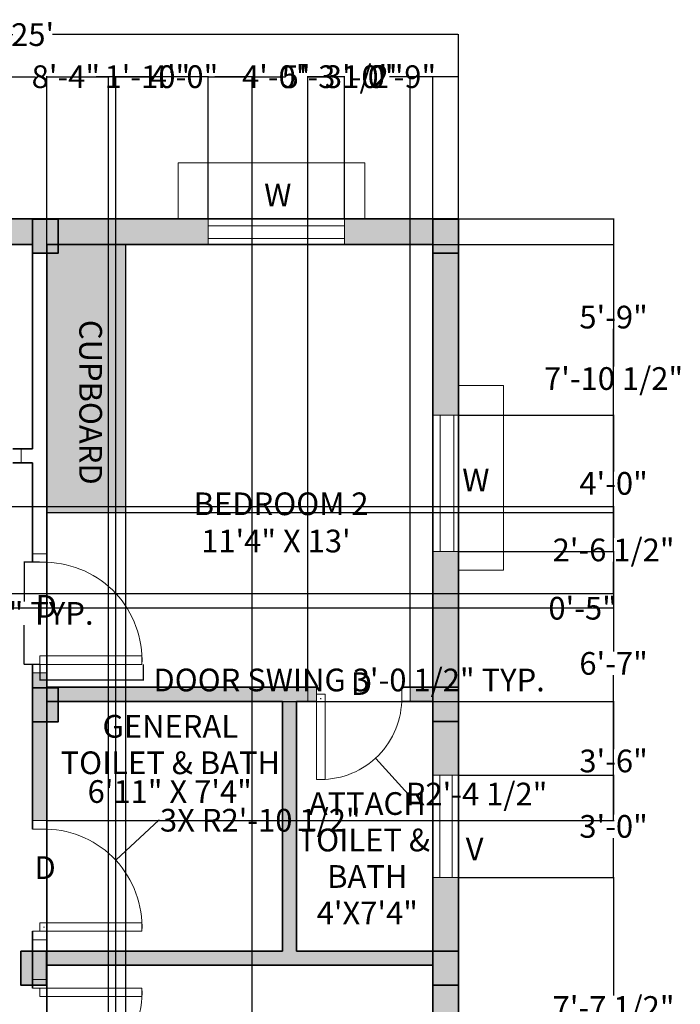
# Model space of a CAD drawing. Units: inches. Extents: x 374 to 1054, y -870 to -188.
# Tile 3 of 3: x 601 to 834, y -535 to -188. Entities that reach past the tile are written whole.
import ezdxf
from ezdxf.enums import TextEntityAlignment as Align

# ---------------------------------------------------------------- set-up
doc = ezdxf.new("R2010")
doc.units = ezdxf.units.IN
doc.header["$MEASUREMENT"] = 0
for name, color, linetype, lineweight, true_color in [('A-ANNO-DIMS', 244, 'Continuous', 18, 0x991b1e), ('A-AREA-IDEN', 116, 'Continuous', 18, 0x136734), ('A-WALL-PATT', 116, 'Continuous', 13, 0x136734)]:
    doc.layers.add(name, color=color, linetype=linetype, lineweight=lineweight, true_color=true_color)
for name, color, linetype, lineweight in [('A-ANNO-TEXT', 7, 'Continuous', 18), ('A-COLS', 1, 'Continuous', 35), ('A-DOOR', 4, 'Continuous', 18), ('A-FLOR-CASE', 8, 'Continuous', 25), ('A-FLOR-CASE-PATT', 8, 'Continuous', 13), ('A-GLAZ', 4, 'Continuous', 18), ('A-GLAZ-PROJ', 4, 'Continuous', 13), ('A-WALL', 7, 'Continuous', 35)]:
    doc.layers.add(name, color=color, linetype=linetype, lineweight=lineweight)
doc.styles.get("Standard").update_dxf_attribs({"font": 'arial.ttf'})
doc.dimstyles.get("Standard").update_dxf_attribs({"dimtxt": 8, "dimasz": 0.18, "dimexe": 0.18, "dimexo": 0.0625, "dimgap": 0.09, "dimtad": 0, "dimtih": 1, "dimtoh": 1, "dimzin": 0, "dimdsep": 46, "dimlunit": 3, "dimtxsty": 'Standard', "dimcen": 0.09, "dimadec": 0, "dimazin": 0, "dimtfac": 1, "dimtofl": 0, "dimtmove": 0, "dimatfit": 3, "dimfxl": 1, "dimtolj": 1, "dimtzin": 0, "dimarcsym": 0})

# ---------------------------------------------------------------- blocks, each defined once
blk = doc.blocks.new('*D1')
at = {"layer": 'A-ANNO-DIMS', "color": 0, "lineweight": -2, "transparency": 16777216}
for p, q in [((455.9, -257.88), (455.9, -192.83)), ((456.08, -193.01), (598.96, -193.01)), ((755.72, -193.01), (612.85, -193.01)), ((755.9, -257.88), (755.9, -192.83))]:
    blk.add_line(p, q, dxfattribs=at)
at = {"layer": 'A-ANNO-DIMS', "color": 0, "transparency": 16777216}
for points in [[(456.08, -192.98), (456.08, -193.04), (455.9, -193.01)], [(755.72, -192.98), (755.72, -193.04), (755.9, -193.01)]]:
    blk.add_solid(points, dxfattribs=at)
at = {"layer": 'Defpoints', "color": 0, "transparency": 16777216}
for p in [(755.9, -193.01), (455.9, -257.94), (755.9, -257.94)]:
    blk.add_point(p, dxfattribs=at)
at = {"layer": 'A-ANNO-DIMS', "color": 0, "transparency": 16777216, "insert": (605.9, -193.01), "char_height": 8, "attachment_point": 5}
blk.add_mtext("\\A1;25'", dxfattribs=at)
blk = doc.blocks.new('COL-12X9')
h = blk.add_hatch(color=256)
h.dxf.hatch_style = 1
h.paths.add_polyline_path([(6, 4.5), (-6, 4.5), (-6, -4.5), (6, -4.5)])
blk.add_lwpolyline([(-6, 4.5), (6, 4.5), (6, -4.5), (-6, -4.5)], close=True)
blk = doc.blocks.new('DOOR-SWING-36')
blk.add_lwpolyline([(0, 0), (-3, 0), (-3, 36), (0, 36)], close=True)
blk.add_arc((-1.5, 1.52), 34.51, 87.5091, 178.3707)
blk = doc.blocks.new('*D8')
at = {"layer": 'A-ANNO-DIMS', "color": 0, "lineweight": -2, "transparency": 16777216}
for p, q in [((608.4, -415), (608.4, -420.58)), ((644.81, -415), (644.81, -420.58)), ((608.58, -420.4), (644.63, -420.4)), ((644.81, -420.4), (644.99, -420.4))]:
    blk.add_line(p, q, dxfattribs=at)
at = {"layer": 'A-ANNO-DIMS', "color": 0, "transparency": 16777216}
for points in [[(608.58, -420.37), (608.58, -420.43), (608.4, -420.4)], [(644.63, -420.37), (644.63, -420.43), (644.81, -420.4)]]:
    blk.add_solid(points, dxfattribs=at)
at = {"layer": 'Defpoints', "color": 0, "transparency": 16777216}
for p in [(608.4, -414.94), (644.81, -414.94), (644.81, -420.4)]:
    blk.add_point(p, dxfattribs=at)
at = {"layer": 'A-ANNO-DIMS', "color": 0, "transparency": 16777216, "insert": (717.38, -420.4), "char_height": 8, "attachment_point": 5}
blk.add_mtext('\\A1;DOOR SWING 3\'-0 1/2" TYP.', dxfattribs=at)
blk = doc.blocks.new('*D9')
at = {"layer": 'A-ANNO-DIMS', "color": 0, "lineweight": -2, "transparency": 16777216}
for p, q in [((608.34, -378.94), (602.76, -378.94)), ((602.94, -379.12), (602.94, -392.76)), ((602.94, -414.76), (602.94, -401.12)), ((608.34, -414.94), (602.76, -414.94))]:
    blk.add_line(p, q, dxfattribs=at)
at = {"layer": 'A-ANNO-DIMS', "color": 0, "transparency": 16777216}
for points in [[(602.91, -379.12), (602.97, -379.12), (602.94, -378.94)], [(602.91, -414.76), (602.97, -414.76), (602.94, -414.94)]]:
    blk.add_solid(points, dxfattribs=at)
at = {"layer": 'Defpoints', "color": 0, "transparency": 16777216}
for p in [(608.4, -378.94), (602.94, -414.94), (608.4, -414.94)]:
    blk.add_point(p, dxfattribs=at)
at = {"layer": 'A-ANNO-DIMS', "color": 0, "transparency": 16777216, "insert": (602.94, -396.94), "char_height": 8, "attachment_point": 5}
blk.add_mtext('\\A1;3\'-0" TYP.', dxfattribs=at)
blk = doc.blocks.new('*D14')
at = {"layer": 'A-ANNO-DIMS', "color": 0, "lineweight": -2, "transparency": 16777216}
for p, q in [((567.48, -257.88), (567.48, -207.66)), ((567.66, -207.84), (606.87, -207.84)), ((667.53, -207.84), (628.32, -207.84)), ((667.71, -257.88), (667.71, -207.66))]:
    blk.add_line(p, q, dxfattribs=at)
at = {"layer": 'A-ANNO-DIMS', "color": 0, "transparency": 16777216}
for points in [[(567.66, -207.81), (567.66, -207.87), (567.48, -207.84)], [(667.53, -207.81), (667.53, -207.87), (667.71, -207.84)]]:
    blk.add_solid(points, dxfattribs=at)
at = {"layer": 'Defpoints', "color": 0, "transparency": 16777216}
for p in [(667.71, -207.84), (567.48, -257.94), (667.71, -257.94)]:
    blk.add_point(p, dxfattribs=at)
at = {"layer": 'A-ANNO-DIMS', "color": 0, "transparency": 16777216, "insert": (617.6, -207.84), "char_height": 8, "attachment_point": 5}
blk.add_mtext('\\A1;8\'-4"', dxfattribs=at)
blk = doc.blocks.new('*D15')
at = {"layer": 'A-ANNO-DIMS', "color": 0, "lineweight": -2, "transparency": 16777216}
for p, q in [((667.71, -257.88), (667.71, -207.66)), ((667.89, -207.84), (680.83, -207.84)), ((715.53, -207.84), (702.59, -207.84)), ((715.71, -257.88), (715.71, -207.66))]:
    blk.add_line(p, q, dxfattribs=at)
at = {"layer": 'A-ANNO-DIMS', "color": 0, "transparency": 16777216}
for points in [[(667.89, -207.81), (667.89, -207.87), (667.71, -207.84)], [(715.53, -207.81), (715.53, -207.87), (715.71, -207.84)]]:
    blk.add_solid(points, dxfattribs=at)
at = {"layer": 'Defpoints', "color": 0, "transparency": 16777216}
for p in [(715.71, -207.84), (667.71, -257.94), (715.71, -257.94)]:
    blk.add_point(p, dxfattribs=at)
at = {"layer": 'A-ANNO-DIMS', "color": 0, "transparency": 16777216, "insert": (691.71, -207.84), "char_height": 8, "attachment_point": 5}
blk.add_mtext('\\A1;4\'-0"', dxfattribs=at)
blk = doc.blocks.new('*D24')
at = {"layer": 'A-ANNO-DIMS', "color": 0, "lineweight": -2, "transparency": 16777216}
for p, q in [((746.9, -207.84), (746.72, -207.84)), ((746.9, -266.88), (746.9, -207.66)), ((755.72, -207.84), (747.08, -207.84)), ((755.9, -257.88), (755.9, -207.66))]:
    blk.add_line(p, q, dxfattribs=at)
at = {"layer": 'A-ANNO-DIMS', "color": 0, "transparency": 16777216}
for points in [[(747.08, -207.81), (747.08, -207.87), (746.9, -207.84)], [(755.72, -207.81), (755.72, -207.87), (755.9, -207.84)]]:
    blk.add_solid(points, dxfattribs=at)
at = {"layer": 'Defpoints', "color": 0, "transparency": 16777216}
for p in [(746.9, -207.84), (755.9, -257.94), (746.9, -266.94)]:
    blk.add_point(p, dxfattribs=at)
at = {"layer": 'A-ANNO-DIMS', "color": 0, "transparency": 16777216, "insert": (736, -207.84), "char_height": 8, "attachment_point": 5}
blk.add_mtext('\\A1;0\'-9"', dxfattribs=at)
blk = doc.blocks.new('*D25')
at = {"layer": 'A-ANNO-DIMS', "color": 0, "lineweight": -2, "transparency": 16777216}
for p, q in [((541.93, -389.94), (810.73, -389.94)), ((810.55, -390.12), (810.55, -394.76)), ((541.92, -394.94), (810.73, -394.94)), ((810.55, -395.12), (810.37, -395.12)), ((810.55, -394.94), (810.55, -395.12))]:
    blk.add_line(p, q, dxfattribs=at)
at = {"layer": 'A-ANNO-DIMS', "color": 0, "transparency": 16777216}
for points in [[(810.52, -390.12), (810.58, -390.12), (810.55, -389.94)], [(810.52, -394.76), (810.58, -394.76), (810.55, -394.94)]]:
    blk.add_solid(points, dxfattribs=at)
at = {"layer": 'Defpoints', "color": 0, "transparency": 16777216}
for p in [(541.86, -389.94), (541.86, -394.94), (810.55, -394.94)]:
    blk.add_point(p, dxfattribs=at)
at = {"layer": 'A-ANNO-DIMS', "color": 0, "transparency": 16777216, "insert": (799.65, -395.12), "char_height": 8, "attachment_point": 5}
blk.add_mtext('\\A1;0\'-5"', dxfattribs=at)
blk = doc.blocks.new('*D26')
at = {"layer": 'A-ANNO-DIMS', "color": 0, "lineweight": -2, "transparency": 16777216}
for p, q in [((755.97, -257.94), (810.73, -257.94)), ((810.55, -258.12), (810.55, -288.36)), ((810.55, -326.96), (810.55, -296.71)), ((755.97, -327.14), (810.73, -327.14))]:
    blk.add_line(p, q, dxfattribs=at)
at = {"layer": 'A-ANNO-DIMS', "color": 0, "transparency": 16777216}
for points in [[(810.52, -258.12), (810.58, -258.12), (810.55, -257.94)], [(810.52, -326.96), (810.58, -326.96), (810.55, -327.14)]]:
    blk.add_solid(points, dxfattribs=at)
at = {"layer": 'Defpoints', "color": 0, "transparency": 16777216}
for p in [(755.9, -257.94), (755.9, -327.14), (810.55, -327.14)]:
    blk.add_point(p, dxfattribs=at)
at = {"layer": 'A-ANNO-DIMS', "color": 0, "transparency": 16777216, "insert": (810.55, -292.54), "char_height": 8, "attachment_point": 5}
blk.add_mtext('\\A1;5\'-9"', dxfattribs=at)
blk = doc.blocks.new('*D27')
at = {"layer": 'A-ANNO-DIMS', "color": 0, "lineweight": -2, "transparency": 16777216}
for p, q in [((755.97, -327.14), (810.73, -327.14)), ((810.55, -327.32), (810.55, -346.96)), ((810.55, -374.96), (810.55, -355.31)), ((755.97, -375.14), (810.73, -375.14))]:
    blk.add_line(p, q, dxfattribs=at)
at = {"layer": 'A-ANNO-DIMS', "color": 0, "transparency": 16777216}
for points in [[(810.52, -327.32), (810.58, -327.32), (810.55, -327.14)], [(810.52, -374.96), (810.58, -374.96), (810.55, -375.14)]]:
    blk.add_solid(points, dxfattribs=at)
at = {"layer": 'Defpoints', "color": 0, "transparency": 16777216}
for p in [(755.9, -327.14), (755.9, -375.14), (810.55, -375.14)]:
    blk.add_point(p, dxfattribs=at)
at = {"layer": 'A-ANNO-DIMS', "color": 0, "transparency": 16777216, "insert": (810.55, -351.14), "char_height": 8, "attachment_point": 5}
blk.add_mtext('\\A1;4\'-0"', dxfattribs=at)
blk = doc.blocks.new('*D28')
at = {"layer": 'A-ANNO-DIMS', "color": 0, "lineweight": -2, "transparency": 16777216}
for p, q in [((755.97, -375.14), (810.73, -375.14)), ((810.55, -375.32), (810.55, -410.39)), ((810.55, -453.81), (810.55, -418.74)), ((755.97, -453.99), (810.73, -453.99))]:
    blk.add_line(p, q, dxfattribs=at)
at = {"layer": 'A-ANNO-DIMS', "color": 0, "transparency": 16777216}
for points in [[(810.52, -375.32), (810.58, -375.32), (810.55, -375.14)], [(810.52, -453.81), (810.58, -453.81), (810.55, -453.99)]]:
    blk.add_solid(points, dxfattribs=at)
at = {"layer": 'Defpoints', "color": 0, "transparency": 16777216}
for p in [(755.9, -375.14), (755.9, -453.99), (810.55, -453.99)]:
    blk.add_point(p, dxfattribs=at)
at = {"layer": 'A-ANNO-DIMS', "color": 0, "transparency": 16777216, "insert": (810.55, -414.57), "char_height": 8, "attachment_point": 5}
blk.add_mtext('\\A1;6\'-7"', dxfattribs=at)
blk = doc.blocks.new('*D29')
at = {"layer": 'A-ANNO-DIMS', "color": 0, "lineweight": -2, "transparency": 16777216}
for p, q in [((755.97, -453.99), (810.73, -453.99)), ((810.55, -454.17), (810.55, -467.82)), ((810.55, -489.81), (810.55, -476.17)), ((755.97, -489.99), (810.73, -489.99))]:
    blk.add_line(p, q, dxfattribs=at)
at = {"layer": 'A-ANNO-DIMS', "color": 0, "transparency": 16777216}
for points in [[(810.52, -454.17), (810.58, -454.17), (810.55, -453.99)], [(810.52, -489.81), (810.58, -489.81), (810.55, -489.99)]]:
    blk.add_solid(points, dxfattribs=at)
at = {"layer": 'Defpoints', "color": 0, "transparency": 16777216}
for p in [(755.9, -453.99), (755.9, -489.99), (810.55, -489.99)]:
    blk.add_point(p, dxfattribs=at)
at = {"layer": 'A-ANNO-DIMS', "color": 0, "transparency": 16777216, "insert": (810.55, -471.99), "char_height": 8, "attachment_point": 5}
blk.add_mtext('\\A1;3\'-0"', dxfattribs=at)
blk = doc.blocks.new('*D30')
at = {"layer": 'A-ANNO-DIMS', "color": 0, "lineweight": -2, "transparency": 16777216}
for p, q in [((755.97, -489.99), (810.73, -489.99)), ((810.55, -490.17), (810.55, -531.58)), ((810.55, -581.43), (810.55, -540.03)), ((755.97, -581.61), (810.73, -581.61))]:
    blk.add_line(p, q, dxfattribs=at)
at = {"layer": 'A-ANNO-DIMS', "color": 0, "transparency": 16777216}
for points in [[(810.52, -490.17), (810.58, -490.17), (810.55, -489.99)], [(810.52, -581.43), (810.58, -581.43), (810.55, -581.61)]]:
    blk.add_solid(points, dxfattribs=at)
at = {"layer": 'Defpoints', "color": 0, "transparency": 16777216}
for p in [(755.9, -489.99), (755.9, -581.61), (810.55, -581.61)]:
    blk.add_point(p, dxfattribs=at)
at = {"layer": 'A-ANNO-DIMS', "color": 0, "transparency": 16777216, "insert": (810.55, -535.8), "char_height": 8, "attachment_point": 5}
blk.add_mtext('\\A1;7\'-7 1/2"', dxfattribs=at)
blk = doc.blocks.new('*D35')
at = {"layer": 'A-ANNO-DIMS', "color": 0, "lineweight": -2, "transparency": 16777216}
for p, q in [((610.9, -361.5), (610.9, -822.55)), ((638.56, -361.5), (638.56, -822.55)), ((611.08, -822.37), (638.38, -822.37)), ((638.56, -822.37), (638.74, -822.37))]:
    blk.add_line(p, q, dxfattribs=at)
at = {"layer": 'A-ANNO-DIMS', "color": 0, "transparency": 16777216}
for points in [[(611.08, -822.34), (611.08, -822.4), (610.9, -822.37)], [(638.38, -822.34), (638.38, -822.4), (638.56, -822.37)]]:
    blk.add_solid(points, dxfattribs=at)
at = {"layer": 'Defpoints', "color": 0, "transparency": 16777216}
for p in [(610.9, -361.44), (638.56, -361.44), (638.56, -822.37)]:
    blk.add_point(p, dxfattribs=at)
at = {"layer": 'A-ANNO-DIMS', "color": 0, "transparency": 16777216, "insert": (658.85, -822.37), "char_height": 8, "attachment_point": 5}
blk.add_mtext('\\A1;2\'-3 1/2"', dxfattribs=at)
blk = doc.blocks.new('*D36')
at = {"layer": 'A-ANNO-DIMS', "color": 0, "lineweight": -2, "transparency": 16777216}
for p, q in [((638.63, -266.94), (810.73, -266.94)), ((810.55, -267.12), (810.55, -309.96)), ((810.55, -361.26), (810.55, -318.41)), ((638.63, -361.44), (810.73, -361.44))]:
    blk.add_line(p, q, dxfattribs=at)
at = {"layer": 'A-ANNO-DIMS', "color": 0, "transparency": 16777216}
for points in [[(810.52, -267.12), (810.58, -267.12), (810.55, -266.94)], [(810.52, -361.26), (810.58, -361.26), (810.55, -361.44)]]:
    blk.add_solid(points, dxfattribs=at)
at = {"layer": 'Defpoints', "color": 0, "transparency": 16777216}
for p in [(638.56, -266.94), (810.55, -266.94), (638.56, -361.44)]:
    blk.add_point(p, dxfattribs=at)
at = {"layer": 'A-ANNO-DIMS', "color": 0, "transparency": 16777216, "insert": (810.55, -314.19), "char_height": 8, "attachment_point": 5}
blk.add_mtext('\\A1;7\'-10 1/2"', dxfattribs=at)
blk = doc.blocks.new('*D37')
at = {"layer": 'A-ANNO-DIMS', "color": 0, "lineweight": -2, "transparency": 16777216}
for p, q in [((610.9, -588.25), (610.9, -207.66)), ((611.08, -207.84), (632.5, -207.84)), ((632.68, -588.25), (632.68, -207.66)), ((632.68, -207.84), (632.86, -207.84))]:
    blk.add_line(p, q, dxfattribs=at)
at = {"layer": 'A-ANNO-DIMS', "color": 0, "transparency": 16777216}
for points in [[(611.08, -207.81), (611.08, -207.87), (610.9, -207.84)], [(632.5, -207.81), (632.5, -207.87), (632.68, -207.84)]]:
    blk.add_solid(points, dxfattribs=at)
at = {"layer": 'Defpoints', "color": 0, "transparency": 16777216}
for p in [(632.68, -207.84), (610.9, -588.31), (632.68, -588.31)]:
    blk.add_point(p, dxfattribs=at)
at = {"layer": 'A-ANNO-DIMS', "color": 0, "transparency": 16777216, "insert": (646.31, -207.84), "char_height": 8, "attachment_point": 5}
blk.add_mtext('\\A1;1\'-10"', dxfattribs=at)
blk = doc.blocks.new('*D43')
at = {"layer": 'A-ANNO-DIMS', "color": 0, "lineweight": -2, "transparency": 16777216}
for p, q in [((635.25, -680.88), (635.25, -207.66)), ((635.43, -207.84), (648.36, -207.84)), ((683.07, -207.84), (670.13, -207.84)), ((683.25, -680.88), (683.25, -207.66))]:
    blk.add_line(p, q, dxfattribs=at)
at = {"layer": 'A-ANNO-DIMS', "color": 0, "transparency": 16777216}
for points in [[(635.43, -207.81), (635.43, -207.87), (635.25, -207.84)], [(683.07, -207.81), (683.07, -207.87), (683.25, -207.84)]]:
    blk.add_solid(points, dxfattribs=at)
at = {"layer": 'Defpoints', "color": 0, "transparency": 16777216}
for p in [(683.25, -207.84), (635.25, -680.94), (683.25, -680.94)]:
    blk.add_point(p, dxfattribs=at)
at = {"layer": 'A-ANNO-DIMS', "color": 0, "transparency": 16777216, "insert": (659.25, -207.84), "char_height": 8, "attachment_point": 5}
blk.add_mtext('\\A1;4\'-0"', dxfattribs=at)
blk = doc.blocks.new('*D44')
at = {"layer": 'A-ANNO-DIMS', "color": 0, "lineweight": -2, "transparency": 16777216}
for p, q in [((683.25, -680.88), (683.25, -207.66)), ((683.43, -207.84), (695.03, -207.84)), ((746.72, -207.84), (735.12, -207.84)), ((746.9, -680.88), (746.9, -207.66))]:
    blk.add_line(p, q, dxfattribs=at)
at = {"layer": 'A-ANNO-DIMS', "color": 0, "transparency": 16777216}
for points in [[(683.43, -207.81), (683.43, -207.87), (683.25, -207.84)], [(746.72, -207.81), (746.72, -207.87), (746.9, -207.84)]]:
    blk.add_solid(points, dxfattribs=at)
at = {"layer": 'Defpoints', "color": 0, "transparency": 16777216}
for p in [(746.9, -207.84), (683.25, -680.94), (746.9, -680.94)]:
    blk.add_point(p, dxfattribs=at)
at = {"layer": 'A-ANNO-DIMS', "color": 0, "transparency": 16777216, "insert": (715.08, -207.84), "char_height": 8, "attachment_point": 5}
blk.add_mtext('\\A1;5\'-3 1/2"', dxfattribs=at)
blk = doc.blocks.new('*D46')
at = {"layer": 'A-ANNO-DIMS', "color": 0, "lineweight": -2, "transparency": 16777216}
for p, q in [((541.95, -359.22), (810.73, -359.22)), ((810.55, -359.4), (810.55, -370.35)), ((810.55, -389.76), (810.55, -378.81)), ((541.93, -389.94), (810.73, -389.94))]:
    blk.add_line(p, q, dxfattribs=at)
at = {"layer": 'A-ANNO-DIMS', "color": 0, "transparency": 16777216}
for points in [[(810.52, -359.4), (810.58, -359.4), (810.55, -359.22)], [(810.52, -389.76), (810.58, -389.76), (810.55, -389.94)]]:
    blk.add_solid(points, dxfattribs=at)
at = {"layer": 'Defpoints', "color": 0, "transparency": 16777216}
for p in [(541.89, -359.22), (541.86, -389.94), (810.55, -389.94)]:
    blk.add_point(p, dxfattribs=at)
at = {"layer": 'A-ANNO-DIMS', "color": 0, "transparency": 16777216, "insert": (810.55, -374.58), "char_height": 8, "attachment_point": 5}
blk.add_mtext('\\A1;2\'-6 1/2"', dxfattribs=at)
blk = doc.blocks.new('*D47')
at = {"layer": 'A-ANNO-DIMS', "color": 0, "lineweight": -2, "transparency": 16777216}
for p, q in [((702.9, -422.88), (702.9, -207.66)), ((703.08, -207.84), (710.18, -207.84)), ((738.72, -207.84), (731.63, -207.84)), ((738.9, -422.88), (738.9, -207.66))]:
    blk.add_line(p, q, dxfattribs=at)
at = {"layer": 'A-ANNO-DIMS', "color": 0, "transparency": 16777216}
for points in [[(703.08, -207.81), (703.08, -207.87), (702.9, -207.84)], [(738.72, -207.81), (738.72, -207.87), (738.9, -207.84)]]:
    blk.add_solid(points, dxfattribs=at)
at = {"layer": 'Defpoints', "color": 0, "transparency": 16777216}
for p in [(738.9, -207.84), (702.9, -422.94), (738.9, -422.94)]:
    blk.add_point(p, dxfattribs=at)
at = {"layer": 'A-ANNO-DIMS', "color": 0, "transparency": 16777216, "insert": (720.9, -207.84), "char_height": 8, "attachment_point": 5}
blk.add_mtext('\\A1;3\'-0"', dxfattribs=at)
blk = doc.blocks.new('*D48')
at = {"layer": 'A-ANNO-DIMS', "color": 0, "lineweight": -2, "transparency": 16777216}
for p, q in [((610.97, -427.94), (810.73, -427.94)), ((810.55, -428.12), (810.55, -444.76)), ((810.55, -469.76), (810.55, -453.12)), ((610.97, -469.94), (810.73, -469.94))]:
    blk.add_line(p, q, dxfattribs=at)
at = {"layer": 'A-ANNO-DIMS', "color": 0, "transparency": 16777216}
for points in [[(810.52, -428.12), (810.58, -428.12), (810.55, -427.94)], [(810.52, -469.76), (810.58, -469.76), (810.55, -469.94)]]:
    blk.add_solid(points, dxfattribs=at)
at = {"layer": 'Defpoints', "color": 0, "transparency": 16777216}
for p in [(610.9, -427.94), (610.9, -469.94), (810.55, -469.94)]:
    blk.add_point(p, dxfattribs=at)
at = {"layer": 'A-ANNO-DIMS', "color": 0, "transparency": 16777216, "insert": (810.55, -448.94), "char_height": 8, "attachment_point": 5}
blk.add_mtext('\\A1;3\'-6"', dxfattribs=at)
blk = doc.blocks.new('*D51')
at = {"layer": 'A-ANNO-DIMS', "color": 0, "lineweight": -2, "transparency": 16777216}
for p, q in [((650.35, -469.82), (635.32, -483.8)), ((650.53, -469.82), (650.35, -469.82)), ((609.83, -507.44), (610.01, -507.44)), ((609.92, -507.53), (609.92, -507.35))]:
    blk.add_line(p, q, dxfattribs=at)
at = {"layer": 'A-ANNO-DIMS', "color": 0, "transparency": 16777216}
blk.add_solid([(635.3, -483.78), (635.34, -483.83), (635.19, -483.93)], dxfattribs=at)
at = {"layer": 'Defpoints', "color": 0, "transparency": 16777216}
for p in [(635.19, -483.93), (609.92, -507.44)]:
    blk.add_point(p, dxfattribs=at)
at = {"layer": 'A-ANNO-DIMS', "color": 0, "transparency": 16777216, "insert": (686.1, -469.82), "char_height": 8, "attachment_point": 5}
blk.add_mtext('\\A1;3X R2\'-10 1/2"', dxfattribs=at)
blk = doc.blocks.new('*D52')
at = {"layer": 'A-ANNO-DIMS', "color": 0, "lineweight": -2, "transparency": 16777216}
for p, q in [((707.31, -426.96), (707.49, -426.96)), ((707.4, -427.05), (707.4, -426.87)), ((738.24, -460.59), (726.8, -448.11)), ((738.42, -460.59), (738.24, -460.59))]:
    blk.add_line(p, q, dxfattribs=at)
at = {"layer": 'A-ANNO-DIMS', "color": 0, "transparency": 16777216}
blk.add_solid([(726.82, -448.09), (726.77, -448.14), (726.67, -447.98)], dxfattribs=at)
at = {"layer": 'Defpoints', "color": 0, "transparency": 16777216}
for p in [(707.4, -426.96), (726.67, -447.98)]:
    blk.add_point(p, dxfattribs=at)
at = {"layer": 'A-ANNO-DIMS', "color": 0, "transparency": 16777216, "insert": (762.29, -460.59), "char_height": 8, "attachment_point": 5}
blk.add_mtext('\\A1;R2\'-4 1/2"', dxfattribs=at)

msp = doc.modelspace()

# ---------------------------------------------------------------- hatches: boundary and pattern name
at = {"layer": 'A-FLOR-CASE-PATT'}
h = msp.add_hatch(dxfattribs=at)
h.set_pattern_fill('AR-HBONE', color=256)
h.paths.add_polyline_path([(638.563, -266.938), (610.905, -266.938), (610.905, -343.938), (610.905, -361.438), (638.563, -361.438)])
h.paths.add_polyline_path([(620.136, -288.822), (620.136, -356.301), (632.553, -356.301), (632.553, -288.822)], flags=24)
h.paths.add_polyline_path([(727.152, -700.465), (727.152, -761.497), (739.414, -761.497), (739.414, -700.465)], flags=9)
h.paths.add_polyline_path([(497.837, -702.053), (512.386, -702.053), (512.386, -690.053), (497.837, -690.053)], flags=9)
h.paths.add_polyline_path([(494.709, -751.886), (551.702, -751.886), (551.702, -739.837), (494.709, -739.837)], flags=9)
h.paths.add_polyline_path([(490.155, -739.027), (556.256, -739.027), (556.256, -727.027), (490.155, -727.027)], flags=9)
h.paths.add_polyline_path([(488.741, -637.8), (555.988, -637.8), (555.988, -625.538), (488.741, -625.538)], flags=9)
h.paths.add_polyline_path([(501.975, -624.968), (542.755, -624.968), (542.755, -612.559), (501.975, -612.559)], flags=9)
h.paths.add_polyline_path([(498.568, -470.79), (565.812, -470.79), (565.812, -458.536), (498.568, -458.536)], flags=9)
h.paths.add_polyline_path([(510.563, -457.965), (553.816, -457.965), (553.816, -445.555), (510.563, -445.555)], flags=9)
h.paths.add_polyline_path([(474.841, -376.354), (525.689, -376.354), (525.689, -364.092), (474.841, -364.092)], flags=9)
h.paths.add_polyline_path([(483.939, -363.488), (516.591, -363.488), (516.591, -351.283), (483.939, -351.283)], flags=9)
h.paths.add_polyline_path([(652.121, -604.662), (719.368, -604.662), (719.368, -592.4), (652.121, -592.4)], flags=9)
h.paths.add_polyline_path([(650.141, -591.831), (721.347, -591.831), (721.347, -579.414), (650.141, -579.414)], flags=9)
h.paths.add_polyline_path([(613.577, -603.955), (613.577, -672.673), (625.995, -672.673), (625.995, -603.955)], flags=9)
h.paths.add_polyline_path([(704.619, -508.492), (742.954, -508.492), (742.954, -496.492), (704.619, -496.492)], flags=9)
h.paths.add_polyline_path([(706.883, -495.641), (740.69, -495.641), (740.69, -483.641), (706.883, -483.641)], flags=9)
h.paths.add_polyline_path([(695.312, -483.057), (752.261, -483.057), (752.261, -470.566), (695.312, -470.566)], flags=9)
h.paths.add_polyline_path([(699.358, -470.143), (748.215, -470.143), (748.215, -457.734), (699.358, -457.734)], flags=9)
h.paths.add_polyline_path([(623.681, -465.885), (684.71, -465.885), (684.71, -453.631), (623.681, -453.631)], flags=9)
h.paths.add_polyline_path([(611.019, -455.848), (697.775, -455.848), (697.775, -443.357), (611.019, -443.357)], flags=9)
h.paths.add_polyline_path([(625.622, -442.934), (683.172, -442.934), (683.172, -430.525), (625.622, -430.525)], flags=9)
at = {"layer": 'A-WALL-PATT'}
h = msp.add_hatch(color=256, dxfattribs=at)
h.dxf.hatch_style = 1
h.paths.add_polyline_path([(667.71, -257.938), (614.905, -257.938), (614.905, -266.938), (667.71, -266.938)])
h.paths.add_polyline_path([(746.905, -257.938), (715.71, -257.938), (715.71, -266.938), (746.905, -266.938)])
h.paths.add_polyline_path([(755.905, -270.034), (746.905, -270.034), (746.905, -327.137), (755.905, -327.137)])
h.paths.add_polyline_path([(755.905, -375.137), (746.905, -375.137), (746.905, -422.975), (755.905, -422.975)])
h.paths.add_polyline_path([(605.905, -257.938), (567.481, -257.938), (567.481, -266.938), (605.905, -266.938)])
h.paths.add_polyline_path([(519.481, -257.938), (464.905, -257.938), (464.905, -266.938), (519.481, -266.938)])
h.paths.add_polyline_path([(464.905, -270.108), (455.905, -270.108), (455.905, -285.73), (464.905, -285.73)])
h.paths.add_polyline_path([(464.905, -343.938), (559.905, -343.938), (559.905, -338.938), (464.905, -338.938), (464.905, -333.73), (455.905, -333.73), (455.905, -353.908), (464.905, -353.908)])
h.paths.add_polyline_path([(464.905, -394.938), (541.859, -394.938), (541.863, -389.942), (536.905, -389.938), (464.905, -389.938), (455.905, -389.908), (455.905, -423.118), (464.905, -423.118)])
h.paths.add_polyline_path([(464.905, -435.118), (455.905, -435.118), (455.905, -449.434), (464.905, -449.434)])
h.paths.add_polyline_path([(464.905, -497.434), (455.905, -497.434), (455.905, -515.926), (464.905, -515.926)])
h.paths.add_polyline_path([(464.905, -527.926), (455.905, -527.926), (455.905, -558.14), (464.905, -558.14)])
h.paths.add_polyline_path([(755.905, -489.995), (746.905, -489.995), (746.905, -515.947), (755.905, -515.947)])
h.paths.add_polyline_path([(755.905, -434.975), (746.905, -434.975), (746.905, -453.995), (755.905, -453.995)])
h.paths.add_polyline_path([(746.905, -422.938), (738.905, -422.938), (738.905, -427.938), (746.905, -427.938)])
h.paths.add_polyline_path([(614.905, -423.118), (614.905, -435.118), (605.905, -435.118), (605.905, -423.118), (605.905, -417.938), (610.905, -417.938), (610.905, -423.118)])
h.paths.add_polyline_path([(610.905, -435.118), (605.905, -435.118), (605.905, -469.938), (610.905, -469.938)])
h.paths.add_polyline_path([(541.859, -515.938), (464.905, -515.938), (464.905, -520.938), (541.859, -520.938)])
h.paths.add_polyline_path([(755.905, -527.947), (746.905, -527.947), (746.905, -581.613), (755.905, -581.613)])
h.paths.add_polyline_path([(755.905, -629.613), (746.905, -629.613), (746.905, -677.938), (755.905, -677.938)])
h.paths.add_polyline_path([(755.905, -689.938), (746.905, -689.938), (746.905, -764.938), (755.905, -764.938)])
h.paths.add_polyline_path([(746.905, -680.938), (683.247, -680.938), (683.247, -689.938), (746.905, -689.938)])
h.paths.add_polyline_path([(743.737, -764.938), (701.105, -764.938), (701.105, -773.938), (743.737, -773.938)])
h.paths.add_polyline_path([(653.105, -764.938), (617.905, -764.938), (617.905, -773.938), (653.105, -773.938)])
h.paths.add_polyline_path([(635.247, -680.938), (614.944, -680.938), (614.944, -689.938), (635.247, -689.938)])
h.paths.add_polyline_path([(610.905, -567.938), (605.905, -567.938), (605.905, -677.938), (610.905, -677.938)])
h.paths.add_polyline_path([(558.905, -680.938), (529.314, -680.938), (529.314, -687.485), (529.314, -689.938), (558.905, -689.938)])
h.paths.add_polyline_path([(481.314, -680.938), (464.905, -680.938), (464.905, -689.938), (481.314, -689.938)])
h.paths.add_polyline_path([(464.905, -606.14), (455.905, -606.14), (455.905, -677.938), (464.905, -677.938)])
h.paths.add_polyline_path([(601.753, -550.416), (613.824, -550.416), (613.824, -538.416), (601.753, -538.416)], flags=9)
h.paths.add_polyline_path([(604.254, -492.526), (616.325, -492.526), (616.325, -480.526), (604.254, -480.526)], flags=9)
h.paths.add_polyline_path([(604.661, -400.451), (616.732, -400.451), (616.732, -388.451), (604.661, -388.451)], flags=9)
h.paths.add_polyline_path([(533.025, -378.901), (545.096, -378.901), (545.096, -366.901), (533.025, -366.901)], flags=9)
h.paths.add_polyline_path([(575.128, -346.003), (587.199, -346.003), (587.199, -334.003), (575.128, -334.003)], flags=9)
h.paths.add_polyline_path([(488.741, -637.8), (555.988, -637.8), (555.988, -625.538), (488.741, -625.538)], flags=9)
h.paths.add_polyline_path([(501.975, -624.968), (542.755, -624.968), (542.755, -612.559), (501.975, -612.559)], flags=9)
h.paths.add_polyline_path([(498.568, -470.79), (565.812, -470.79), (565.812, -458.536), (498.568, -458.536)], flags=9)
h.paths.add_polyline_path([(510.563, -457.965), (553.816, -457.965), (553.816, -445.555), (510.563, -445.555)], flags=9)
h.paths.add_polyline_path([(474.841, -376.354), (525.689, -376.354), (525.689, -364.092), (474.841, -364.092)], flags=9)
h.paths.add_polyline_path([(483.939, -363.488), (516.591, -363.488), (516.591, -351.283), (483.939, -351.283)], flags=9)
h.paths.add_polyline_path([(652.121, -604.662), (719.368, -604.662), (719.368, -592.4), (652.121, -592.4)], flags=9)
h.paths.add_polyline_path([(650.141, -591.831), (721.347, -591.831), (721.347, -579.414), (650.141, -579.414)], flags=9)
h.paths.add_polyline_path([(715.698, -427.661), (727.769, -427.661), (727.769, -415.661), (715.698, -415.661)], flags=9)
h.paths.add_polyline_path([(573.757, -690.34), (585.828, -690.34), (585.828, -678.34), (573.757, -678.34)], flags=9)
h.paths.add_polyline_path([(727.152, -700.465), (727.152, -761.497), (739.414, -761.497), (739.414, -700.465)], flags=9)
h.paths.add_polyline_path([(497.837, -702.053), (512.386, -702.053), (512.386, -690.053), (497.837, -690.053)], flags=9)
h.paths.add_polyline_path([(494.709, -751.886), (551.702, -751.886), (551.702, -739.837), (494.709, -739.837)], flags=9)
h.paths.add_polyline_path([(490.155, -739.027), (556.256, -739.027), (556.256, -727.027), (490.155, -727.027)], flags=9)
h.paths.add_polyline_path([(613.577, -603.955), (613.577, -672.673), (625.995, -672.673), (625.995, -603.955)], flags=9)
h.paths.add_polyline_path([(695.312, -483.057), (752.261, -483.057), (752.261, -470.566), (695.312, -470.566)], flags=9)
h.paths.add_polyline_path([(611.019, -455.848), (697.775, -455.848), (697.775, -443.357), (611.019, -443.357)], flags=9)
h.paths.add_polyline_path([(663.069, -377.631), (720.133, -377.631), (720.133, -365.369), (663.069, -365.369)], flags=9)
h.paths.add_polyline_path([(657.829, -364.537), (729.035, -364.537), (729.035, -352.12), (657.829, -352.12)], flags=9)
h.paths.add_polyline_path([(620.136, -288.822), (620.136, -356.301), (632.553, -356.301), (632.553, -288.822)], flags=9)
h.paths.add_polyline_path([(497.968, -305.851), (548.814, -305.851), (548.814, -293.597), (497.968, -293.597)], flags=9)
h.paths.add_polyline_path([(496.797, -293.026), (549.986, -293.026), (549.986, -280.617), (496.797, -280.617)], flags=9)
h = msp.add_hatch(color=256, dxfattribs=at)
h.dxf.hatch_style = 1
h.paths.add_polyline_path([(705.905, -425.438), (705.905, -422.938), (610.905, -422.938), (610.905, -417.938), (605.905, -417.938), (605.905, -469.938), (610.905, -469.938), (610.905, -435.118), (610.905, -427.938), (693.905, -427.938), (698.905, -427.938), (705.905, -427.938)])
h.paths.add_polyline_path([(715.698, -427.661), (727.769, -427.661), (727.769, -415.661), (715.698, -415.661)], flags=9)
h.paths.add_polyline_path([(573.757, -690.34), (585.828, -690.34), (585.828, -678.34), (573.757, -678.34)], flags=9)
h.paths.add_polyline_path([(601.753, -550.416), (613.824, -550.416), (613.824, -538.416), (601.753, -538.416)], flags=9)
h.paths.add_polyline_path([(604.254, -492.526), (616.325, -492.526), (616.325, -480.526), (604.254, -480.526)], flags=9)
h.paths.add_polyline_path([(604.661, -400.451), (616.732, -400.451), (616.732, -388.451), (604.661, -388.451)], flags=9)
h.paths.add_polyline_path([(533.025, -378.901), (545.096, -378.901), (545.096, -366.901), (533.025, -366.901)], flags=9)
h.paths.add_polyline_path([(575.128, -346.003), (587.199, -346.003), (587.199, -334.003), (575.128, -334.003)], flags=9)
h.paths.add_polyline_path([(727.152, -700.465), (727.152, -761.497), (739.414, -761.497), (739.414, -700.465)], flags=9)
h.paths.add_polyline_path([(497.837, -702.053), (512.386, -702.053), (512.386, -690.053), (497.837, -690.053)], flags=9)
h.paths.add_polyline_path([(494.709, -751.886), (551.702, -751.886), (551.702, -739.837), (494.709, -739.837)], flags=9)
h.paths.add_polyline_path([(490.155, -739.027), (556.256, -739.027), (556.256, -727.027), (490.155, -727.027)], flags=9)
h.paths.add_polyline_path([(488.741, -637.8), (555.988, -637.8), (555.988, -625.538), (488.741, -625.538)], flags=9)
h.paths.add_polyline_path([(501.975, -624.968), (542.755, -624.968), (542.755, -612.559), (501.975, -612.559)], flags=9)
h.paths.add_polyline_path([(498.568, -470.79), (565.812, -470.79), (565.812, -458.536), (498.568, -458.536)], flags=9)
h.paths.add_polyline_path([(510.563, -457.965), (553.816, -457.965), (553.816, -445.555), (510.563, -445.555)], flags=9)
h.paths.add_polyline_path([(474.841, -376.354), (525.689, -376.354), (525.689, -364.092), (474.841, -364.092)], flags=9)
h.paths.add_polyline_path([(483.939, -363.488), (516.591, -363.488), (516.591, -351.283), (483.939, -351.283)], flags=9)
h.paths.add_polyline_path([(652.121, -604.662), (719.368, -604.662), (719.368, -592.4), (652.121, -592.4)], flags=9)
h.paths.add_polyline_path([(650.141, -591.831), (721.347, -591.831), (721.347, -579.414), (650.141, -579.414)], flags=9)
h.paths.add_polyline_path([(613.577, -603.955), (613.577, -672.673), (625.995, -672.673), (625.995, -603.955)], flags=9)
h.paths.add_polyline_path([(704.619, -508.492), (742.954, -508.492), (742.954, -496.492), (704.619, -496.492)], flags=9)
h.paths.add_polyline_path([(706.883, -495.641), (740.69, -495.641), (740.69, -483.641), (706.883, -483.641)], flags=9)
h.paths.add_polyline_path([(695.312, -483.057), (752.261, -483.057), (752.261, -470.566), (695.312, -470.566)], flags=9)
h.paths.add_polyline_path([(699.358, -470.143), (748.215, -470.143), (748.215, -457.734), (699.358, -457.734)], flags=9)
h.paths.add_polyline_path([(623.681, -465.885), (684.71, -465.885), (684.71, -453.631), (623.681, -453.631)], flags=25)
h.paths.add_polyline_path([(611.019, -455.848), (697.775, -455.848), (697.775, -443.357), (611.019, -443.357)], flags=25)
h.paths.add_polyline_path([(625.622, -442.934), (683.172, -442.934), (683.172, -430.525), (625.622, -430.525)], flags=25)
h.paths.add_polyline_path([(663.069, -377.631), (720.133, -377.631), (720.133, -365.369), (663.069, -365.369)], flags=9)
h.paths.add_polyline_path([(657.829, -364.537), (729.035, -364.537), (729.035, -352.12), (657.829, -352.12)], flags=9)
h.paths.add_polyline_path([(620.136, -288.822), (620.136, -356.301), (632.553, -356.301), (632.553, -288.822)], flags=9)
h.paths.add_polyline_path([(497.968, -305.851), (548.814, -305.851), (548.814, -293.597), (497.968, -293.597)], flags=9)
h.paths.add_polyline_path([(496.797, -293.026), (549.986, -293.026), (549.986, -280.617), (496.797, -280.617)], flags=9)
h = msp.add_hatch(color=256, dxfattribs=at)
h.dxf.hatch_style = 1
h.paths.add_polyline_path([(698.905, -427.938), (693.905, -427.938), (693.905, -515.938), (698.905, -515.938)])
h.paths.add_polyline_path([(746.905, -515.938), (698.905, -515.938), (693.905, -515.938), (610.905, -515.938), (610.783, -515.938), (610.783, -520.938), (746.905, -520.938)])
h.paths.add_polyline_path([(695.312, -483.057), (752.261, -483.057), (752.261, -470.566), (695.312, -470.566)], flags=9)
h.paths.add_polyline_path([(611.019, -455.848), (697.775, -455.848), (697.775, -443.357), (611.019, -443.357)], flags=9)

# ---------------------------------------------------------------- linework, layer by layer
at = {"layer": 'A-DOOR'}
for p, q in [((601.905, -338.938), (601.905, -343.938)), ((610.905, -375.938), (605.905, -375.938)), ((610.905, -378.938), (605.905, -378.938)), ((610.905, -414.938), (605.905, -414.938)), ((610.905, -417.938), (605.905, -417.938)), ((702.905, -427.938), (702.905, -422.938)), ((705.905, -427.938), (705.905, -422.938)), ((735.905, -427.938), (735.905, -422.938)), ((738.905, -427.938), (738.905, -422.938)), ((610.905, -469.938), (605.905, -469.938)), ((610.905, -472.938), (605.905, -472.938)), ((610.905, -508.938), (605.905, -508.938)), ((610.905, -511.938), (605.905, -511.938)), ((610.905, -525.938), (605.905, -525.938)), ((610.905, -528.938), (605.905, -528.938))]:
    msp.add_line(p, q, dxfattribs=at)
msp.add_lwpolyline([(705.905, -425.438), (708.905, -425.438), (708.905, -455.438), (705.905, -455.438)], close=True, dxfattribs=at)
msp.add_arc((707.405, -426.961), 28.517, 266.98481, 358.03608, dxfattribs=at)
at = {"layer": 'A-FLOR-CASE'}
for p in [(638.563, -266.938), (610.905, -361.438)]:
    msp.add_line(p, (638.563, -361.438), dxfattribs=at)
at = {"layer": 'A-GLAZ'}
for p, q in [((667.71, -266.938), (667.71, -257.938)), ((715.71, -266.938), (715.71, -257.938)), ((667.71, -260.421), (715.71, -260.421)), ((715.71, -264.841), (667.71, -264.841)), ((755.905, -327.137), (746.905, -327.137)), ((749.481, -327.137), (749.481, -375.137)), ((754.32, -375.137), (754.32, -327.137)), ((755.905, -375.137), (746.905, -375.137)), ((746.905, -453.995), (755.905, -453.995)), ((749.299, -453.995), (749.299, -489.995)), ((753.655, -489.995), (753.655, -453.995)), ((746.905, -489.995), (755.905, -489.995))]:
    msp.add_line(p, q, dxfattribs=at)
at = {"layer": 'A-GLAZ-PROJ'}
for p, q in [((657.14, -257.938), (657.14, -238.231)), ((657.14, -238.231), (722.883, -238.231)), ((722.883, -238.231), (722.883, -257.938)), ((755.905, -316.684), (771.785, -316.684)), ((771.785, -316.684), (771.785, -381.727)), ((771.785, -381.727), (755.905, -381.727))]:
    msp.add_line(p, q, dxfattribs=at)
at = {"layer": 'A-WALL'}
for p, q in [((464.905, -266.938), (605.905, -266.938)), ((605.905, -338.938), (605.905, -266.938)), ((610.905, -343.938), (610.905, -266.938)), ((610.905, -266.938), (746.905, -266.938)), ((746.905, -266.938), (746.905, -422.938)), ((598.905, -338.938), (605.905, -338.938)), ((598.905, -343.938), (605.905, -343.938)), ((605.905, -378.938), (605.905, -343.938)), ((610.905, -378.938), (610.905, -343.938)), ((605.905, -472.938), (605.905, -414.938)), ((610.905, -422.938), (610.905, -414.938)), ((610.905, -422.938), (705.905, -422.938)), ((735.905, -422.938), (746.905, -422.938)), ((610.905, -427.938), (693.905, -427.938)), ((610.905, -472.938), (610.905, -427.938)), ((693.905, -427.938), (693.905, -515.938)), ((698.905, -427.938), (698.905, -515.938)), ((698.905, -427.938), (705.905, -427.938)), ((735.905, -427.938), (746.905, -427.938)), ((746.905, -427.938), (746.905, -515.938)), ((605.905, -528.938), (605.905, -508.938)), ((610.905, -515.938), (610.905, -508.938)), ((610.905, -515.938), (693.905, -515.938)), ((698.905, -515.938), (746.905, -515.938)), ((610.905, -520.938), (746.905, -520.938)), ((610.905, -528.938), (610.905, -520.938)), ((746.905, -520.938), (746.905, -680.938))]:
    msp.add_line(p, q, dxfattribs=at)
msp.add_lwpolyline([(455.905, -257.938), (755.905, -257.938), (755.905, -773.938), (455.905, -773.938)], close=True, dxfattribs=at)

# ---------------------------------------------------------------- block references
at = {"layer": 'A-COLS'}
for p, rotation in [((610.405, -263.99), 269.9999999999994), ((751.405, -264.034), 269.9999999999988), ((610.405, -429.118), 269.9999999999991), ((751.405, -428.975), 269.9999999999988), ((606.283, -521.961), 269.9999999999994), ((751.405, -521.947), 269.9999999999988)]:
    msp.add_blockref('COL-12X9', p, dxfattribs=dict(at, rotation=rotation))
at = {"layer": 'A-DOOR', "rotation": 269.9999999999999}
for p in [(608.405, -414.938), (608.405, -508.938)]:
    msp.add_blockref('DOOR-SWING-36', p, dxfattribs=at)
at = {"layer": 'A-DOOR', "extrusion": (0, 0, -1), "zscale": -1, "rotation": 89.99999999999989}
msp.add_blockref('DOOR-SWING-36', (-608.405, -528.938), dxfattribs=at)

# ---------------------------------------------------------------- texts
at = {"layer": 'A-ANNO-TEXT'}
for s, p in [('W', (692.269, -253.573)), ('W', (762.038, -353.966)), ('D', (610.696, -398.451)), ('D', (721.733, -425.661)), ('V', (761.603, -483.926)), ('D', (610.29, -490.526))]:
    msp.add_text(s, height=8, dxfattribs=at).set_placement(p, align=Align.CENTER)
msp.add_text('CUPBOARD', height=8, rotation=270, dxfattribs=at).set_placement((622.342, -322.561), align=Align.CENTER)
at = {"layer": 'A-AREA-IDEN'}
for s, p in [('BEDROOM 2', (693.432, -362.331)), ('11\'4" X 13\'', (691.601, -375.445)), ('GENERAL', (654.397, -440.73)), ('TOILET & BATH', (654.397, -453.581)), ('6\'11" X 7\'4"', (654.196, -463.706)), ('ATTACH', (723.786, -467.939)), ('TOILET & ', (723.786, -480.79)), ('BATH', (723.786, -493.641)), ('4\'X7\'4"', (723.786, -506.492))]:
    msp.add_text(s, height=8, dxfattribs=at).set_placement(p, align=Align.CENTER)

# ---------------------------------------------------------------- dimensions: what is measured, and where the dimension line sits
at = {"layer": 'A-ANNO-DIMS'}
for base, p1, p2, override, picture, middle in [((755.905, -193.005), (455.905, -257.938), (755.905, -257.938), {"dimclrd": 0, "dimclre": 0, "dimclrt": 0}, '*D1', (605.905, -193.005)), ((746.905, -207.841), (683.247, -680.938), (746.905, -680.938), {"dimdec": 1, "dimlfac": 1, "dimrnd": 0, "dimzin": 1, "dimdsep": 46, "dimlunit": 4, "dimfrac": 2}, '*D44', (715.076, -207.841)), ((667.71, -207.841), (567.481, -257.938), (667.71, -257.938), {"dimdec": 1, "dimlfac": 1, "dimrnd": 0, "dimzin": 1, "dimdsep": 46, "dimlunit": 4, "dimfrac": 2}, '*D14', (617.596, -207.841)), ((632.678, -207.841), (610.905, -588.314), (632.678, -588.314), {"dimdec": 1, "dimlfac": 1, "dimrnd": 0, "dimzin": 1, "dimdsep": 46, "dimlunit": 4, "dimfrac": 2}, '*D37', (646.312, -207.841)), ((683.247, -207.841), (635.247, -680.938), (683.247, -680.938), {"dimdec": 1, "dimlfac": 1, "dimrnd": 0, "dimzin": 1, "dimdsep": 46, "dimlunit": 4, "dimfrac": 2}, '*D43', (659.247, -207.841)), ((715.71, -207.841), (667.71, -257.938), (715.71, -257.938), {"dimdec": 1, "dimlfac": 1, "dimrnd": 0, "dimzin": 1, "dimdsep": 46, "dimlunit": 4, "dimfrac": 2}, '*D15', (691.71, -207.841)), ((738.905, -207.841), (702.905, -422.938), (738.905, -422.938), {"dimdec": 1, "dimlfac": 1, "dimrnd": 0, "dimzin": 1, "dimdsep": 46, "dimlunit": 4, "dimfrac": 2}, '*D47', (720.905, -207.841)), ((746.905, -207.841), (755.905, -257.938), (746.905, -266.938), {"dimdec": 1, "dimlfac": 1, "dimrnd": 0, "dimzin": 1, "dimdsep": 46, "dimlunit": 4, "dimfrac": 2}, '*D24', (736.002, -207.841)), ((638.563, -822.366), (610.905, -361.438), (638.563, -361.438), {"dimdec": 1, "dimlfac": 1, "dimrnd": 0, "dimzin": 1, "dimdsep": 46, "dimlunit": 4, "dimfrac": 2}, '*D35', (658.855, -822.366))]:
    dim = msp.add_linear_dim(base=base, p1=p1, p2=p2, dimstyle='Standard', override=override, dxfattribs=at)
    dim.commit()
    dim.dimension.update_dxf_attribs({"geometry": picture, "text_midpoint": middle})
for base, p1, p2, picture, middle in [((810.55, -327.137), (755.905, -257.938), (755.905, -327.137), '*D26', (810.55, -292.537)), ((810.55, -266.938), (638.563, -361.438), (638.563, -266.938), '*D36', (810.55, -314.188)), ((810.55, -375.137), (755.905, -327.137), (755.905, -375.137), '*D27', (810.55, -351.137)), ((810.55, -389.942), (541.891, -359.22), (541.863, -389.942), '*D46', (810.55, -374.581)), ((810.55, -453.995), (755.905, -375.137), (755.905, -453.995), '*D28', (810.55, -414.566)), ((810.55, -394.938), (541.863, -389.942), (541.859, -394.938), '*D25', (799.647, -395.118)), ((810.55, -469.938), (610.905, -427.938), (610.905, -469.938), '*D48', (810.55, -448.938)), ((810.55, -489.995), (755.905, -453.995), (755.905, -489.995), '*D29', (810.55, -471.995)), ((810.55, -581.613), (755.905, -489.995), (755.905, -581.613), '*D30', (810.55, -535.804))]:
    dim = msp.add_linear_dim(base=base, p1=p1, p2=p2, angle=90, dimstyle='Standard', override={"dimdec": 1, "dimlfac": 1, "dimrnd": 0, "dimzin": 1, "dimdsep": 46, "dimlunit": 4, "dimfrac": 2}, dxfattribs=at)
    dim.commit()
    dim.dimension.update_dxf_attribs({"geometry": picture, "text_midpoint": middle})
dim = msp.add_linear_dim(base=(602.945, -414.938), p1=(608.405, -378.938), p2=(608.405, -414.938), angle=270, text='<> TYP.', dimstyle='Standard', override={"dimdec": 1, "dimlfac": 1, "dimrnd": 0, "dimzin": 1, "dimdsep": 46, "dimlunit": 4, "dimfrac": 2}, dxfattribs=at)
dim.commit()
dim.dimension.update_dxf_attribs({"geometry": '*D9', "text_midpoint": (602.945, -396.938)})
dim = msp.add_linear_dim(base=(644.807, -420.398), p1=(608.405, -414.938), p2=(644.807, -414.938), text='DOOR SWING <> TYP.', dimstyle='Standard', override={"dimdec": 1, "dimlfac": 1, "dimrnd": 0, "dimzin": 1, "dimdsep": 46, "dimlunit": 4, "dimfrac": 2}, dxfattribs=at)
dim.commit()
dim.dimension.update_dxf_attribs({"geometry": '*D8', "text_midpoint": (717.385, -420.398)})
dim = msp.add_radius_dim(center=(707.405, -426.961), mpoint=(726.674, -447.982), dimstyle='Standard', override={"dimdec": 1, "dimlfac": 1, "dimrnd": 0, "dimzin": 1, "dimdsep": 46, "dimlunit": 4, "dimfrac": 2}, dxfattribs=at)
dim.commit()
dim.dimension.update_dxf_attribs({"geometry": '*D52', "text_midpoint": (762.287, -460.595), "dimtype": 164})
dim = msp.add_radius_dim(center=(609.923, -507.438), mpoint=(635.19, -483.926), text='3X <>', dimstyle='Standard', override={"dimdec": 1, "dimlfac": 1, "dimrnd": 0, "dimzin": 1, "dimdsep": 46, "dimlunit": 4, "dimfrac": 2}, dxfattribs=at)
dim.commit()
dim.dimension.update_dxf_attribs({"geometry": '*D51', "text_midpoint": (686.102, -469.819), "dimtype": 164})

doc.saveas('drawing.dxf')
